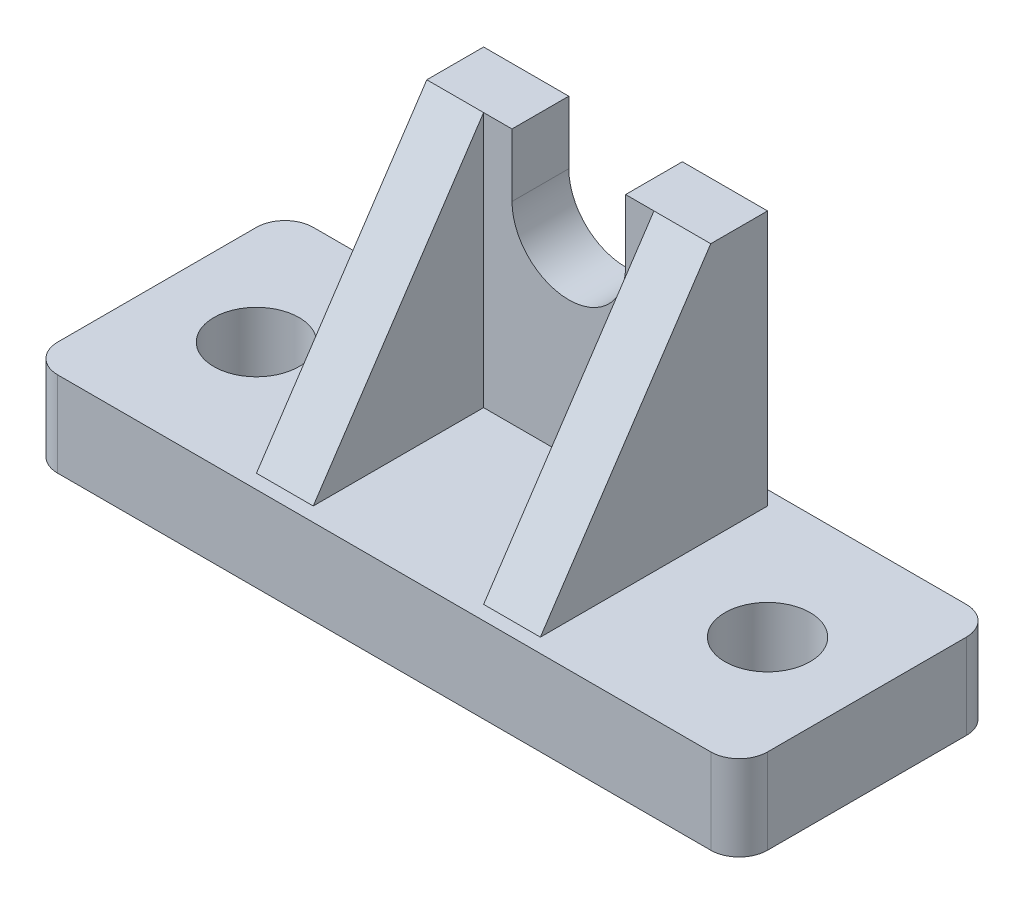
ISO-10303-21;
HEADER;
FILE_DESCRIPTION(('STEP AP214'),'2;1');
FILE_NAME('part.step','',(''),(''),'','','');
FILE_SCHEMA(('AUTOMOTIVE_DESIGN { 1 0 10303 214 1 1 1 1 }'));
ENDSEC;
DATA;
#1=APPLICATION_CONTEXT('core data for automotive mechanical design processes');
#2=APPLICATION_PROTOCOL_DEFINITION('international standard','automotive_design',2000,#1);
#3=PRODUCT_CONTEXT('',#1,'mechanical');
#4=PRODUCT('Part','Part','',(#3));
#5=PRODUCT_RELATED_PRODUCT_CATEGORY('part','',(#4));
#6=PRODUCT_DEFINITION_FORMATION('','',#4);
#7=PRODUCT_DEFINITION_CONTEXT('part definition',#1,'design');
#8=PRODUCT_DEFINITION('design','',#6,#7);
#9=PRODUCT_DEFINITION_SHAPE('','',#8);
#10=(LENGTH_UNIT() NAMED_UNIT(*) SI_UNIT(.MILLI.,.METRE.));
#11=(NAMED_UNIT(*) PLANE_ANGLE_UNIT() SI_UNIT($,.RADIAN.));
#12=(NAMED_UNIT(*) SI_UNIT($,.STERADIAN.) SOLID_ANGLE_UNIT());
#13=UNCERTAINTY_MEASURE_WITH_UNIT(LENGTH_MEASURE(1.E-05),#10,'distance_accuracy_value','');
#14=(GEOMETRIC_REPRESENTATION_CONTEXT(3) GLOBAL_UNCERTAINTY_ASSIGNED_CONTEXT((#13)) GLOBAL_UNIT_ASSIGNED_CONTEXT((#10,
#11,#12)) REPRESENTATION_CONTEXT('',''));
#15=CARTESIAN_POINT('',(0.,0.,0.));
#16=DIRECTION('',(0.,0.,1.));
#17=DIRECTION('',(1.,0.,0.));
#18=AXIS2_PLACEMENT_3D('',#15,#16,#17);
#19=CARTESIAN_POINT('',(50.,48.,-8.));
#20=DIRECTION('',(0.,-0.554700196225229,-0.832050294337844));
#21=DIRECTION('',(0.,0.832050294337844,-0.554700196225229));
#22=AXIS2_PLACEMENT_3D('',#19,#20,#21);
#23=PLANE('',#22);
#24=DIRECTION('',(0.,-0.832050294337844,0.554700196225229));
#25=VECTOR('',#24,1.);
#26=CARTESIAN_POINT('',(-12.,12.,16.));
#27=LINE('',#26,#25);
#28=CARTESIAN_POINT('',(-12.,48.,-8.));
#29=VERTEX_POINT('',#28);
#30=CARTESIAN_POINT('',(-12.,12.,16.));
#31=VERTEX_POINT('',#30);
#32=EDGE_CURVE('E181',#29,#31,#27,.T.);
#33=ORIENTED_EDGE('',*,*,#32,.F.);
#34=DIRECTION('',(-1.,0.,0.));
#35=VECTOR('',#34,1.);
#36=CARTESIAN_POINT('',(50.,48.,-8.));
#37=LINE('',#36,#35);
#38=CARTESIAN_POINT('',(-20.,48.,-8.));
#39=VERTEX_POINT('',#38);
#40=EDGE_CURVE('E197',#29,#39,#37,.T.);
#41=ORIENTED_EDGE('',*,*,#40,.T.);
#42=DIRECTION('',(0.,-0.832050294337844,0.554700196225229));
#43=VECTOR('',#42,1.);
#44=CARTESIAN_POINT('',(-20.,48.,-8.));
#45=LINE('',#44,#43);
#46=CARTESIAN_POINT('',(-20.,12.,16.));
#47=VERTEX_POINT('',#46);
#48=EDGE_CURVE('E194',#39,#47,#45,.T.);
#49=ORIENTED_EDGE('',*,*,#48,.T.);
#50=DIRECTION('',(-1.,0.,0.));
#51=VECTOR('',#50,1.);
#52=CARTESIAN_POINT('',(50.,12.,16.));
#53=LINE('',#52,#51);
#54=EDGE_CURVE('E178',#31,#47,#53,.T.);
#55=ORIENTED_EDGE('',*,*,#54,.F.);
#56=EDGE_LOOP('',(#33,#41,#49,#55));
#57=FACE_BOUND('',#56,.T.);
#58=ADVANCED_FACE('F39',(#57),#23,.F.);
#59=CARTESIAN_POINT('',(50.,12.,18.));
#60=DIRECTION('',(0.,-1.,0.));
#61=DIRECTION('',(1.,0.,0.));
#62=AXIS2_PLACEMENT_3D('',#59,#60,#61);
#63=PLANE('',#62);
#64=DIRECTION('',(-1.,0.,0.));
#65=VECTOR('',#64,1.);
#66=CARTESIAN_POINT('',(50.,12.,18.));
#67=LINE('',#66,#65);
#68=CARTESIAN_POINT('',(46.,12.,18.));
#69=VERTEX_POINT('',#68);
#70=CARTESIAN_POINT('',(-46.,12.,18.));
#71=VERTEX_POINT('',#70);
#72=EDGE_CURVE('E297',#69,#71,#67,.T.);
#73=ORIENTED_EDGE('',*,*,#72,.F.);
#74=CARTESIAN_POINT('',(46.,12.,14.));
#75=DIRECTION('',(0.,-1.,0.));
#76=DIRECTION('',(1.,0.,0.));
#77=AXIS2_PLACEMENT_3D('',#74,#75,#76);
#78=CIRCLE('',#77,4.);
#79=CARTESIAN_POINT('',(50.,12.,14.));
#80=VERTEX_POINT('',#79);
#81=EDGE_CURVE('E62',#80,#69,#78,.T.);
#82=ORIENTED_EDGE('',*,*,#81,.F.);
#83=DIRECTION('',(0.,0.,-1.));
#84=VECTOR('',#83,1.);
#85=CARTESIAN_POINT('',(50.,12.,18.));
#86=LINE('',#85,#84);
#87=CARTESIAN_POINT('',(50.,12.,-14.));
#88=VERTEX_POINT('',#87);
#89=EDGE_CURVE('E309',#80,#88,#86,.T.);
#90=ORIENTED_EDGE('',*,*,#89,.T.);
#91=CARTESIAN_POINT('',(46.,12.,-14.));
#92=DIRECTION('',(0.,-1.,0.));
#93=DIRECTION('',(-1.,0.,0.));
#94=AXIS2_PLACEMENT_3D('',#91,#92,#93);
#95=CIRCLE('',#94,4.);
#96=CARTESIAN_POINT('',(46.,12.,-18.));
#97=VERTEX_POINT('',#96);
#98=EDGE_CURVE('E268',#97,#88,#95,.T.);
#99=ORIENTED_EDGE('',*,*,#98,.F.);
#100=DIRECTION('',(-1.,0.,0.));
#101=VECTOR('',#100,1.);
#102=CARTESIAN_POINT('',(50.,12.,-18.));
#103=LINE('',#102,#101);
#104=CARTESIAN_POINT('',(-46.,12.,-18.));
#105=VERTEX_POINT('',#104);
#106=EDGE_CURVE('E299',#97,#105,#103,.T.);
#107=ORIENTED_EDGE('',*,*,#106,.T.);
#108=CARTESIAN_POINT('',(-46.,12.,-14.));
#109=DIRECTION('',(0.,-1.,0.));
#110=DIRECTION('',(1.,0.,0.));
#111=AXIS2_PLACEMENT_3D('',#108,#109,#110);
#112=CIRCLE('',#111,4.);
#113=CARTESIAN_POINT('',(-50.,12.,-14.));
#114=VERTEX_POINT('',#113);
#115=EDGE_CURVE('E262',#114,#105,#112,.T.);
#116=ORIENTED_EDGE('',*,*,#115,.F.);
#117=DIRECTION('',(0.,0.,-1.));
#118=VECTOR('',#117,1.);
#119=CARTESIAN_POINT('',(-50.,12.,18.));
#120=LINE('',#119,#118);
#121=CARTESIAN_POINT('',(-50.,12.,14.));
#122=VERTEX_POINT('',#121);
#123=EDGE_CURVE('E307',#122,#114,#120,.T.);
#124=ORIENTED_EDGE('',*,*,#123,.F.);
#125=CARTESIAN_POINT('',(-46.,12.,14.));
#126=DIRECTION('',(0.,-1.,0.));
#127=DIRECTION('',(-1.,0.,0.));
#128=AXIS2_PLACEMENT_3D('',#125,#126,#127);
#129=CIRCLE('',#128,4.);
#130=EDGE_CURVE('E267',#71,#122,#129,.T.);
#131=ORIENTED_EDGE('',*,*,#130,.F.);
#132=EDGE_LOOP('',(#73,#82,#90,#99,#107,#116,#124,#131));
#133=FACE_BOUND('',#132,.T.);
#134=CARTESIAN_POINT('',(36.,12.,0.));
#135=DIRECTION('',(0.,1.,0.));
#136=DIRECTION('',(1.,0.,0.));
#137=AXIS2_PLACEMENT_3D('',#134,#135,#136);
#138=CIRCLE('',#137,6.);
#139=CARTESIAN_POINT('',(42.,12.,0.));
#140=VERTEX_POINT('',#139);
#141=EDGE_CURVE('E235',#140,#140,#138,.T.);
#142=ORIENTED_EDGE('',*,*,#141,.F.);
#143=EDGE_LOOP('',(#142));
#144=FACE_BOUND('',#143,.T.);
#145=CARTESIAN_POINT('',(-36.,12.,0.));
#146=DIRECTION('',(0.,1.,0.));
#147=DIRECTION('',(-1.,0.,0.));
#148=AXIS2_PLACEMENT_3D('',#145,#146,#147);
#149=CIRCLE('',#148,6.);
#150=CARTESIAN_POINT('',(-42.,12.,0.));
#151=VERTEX_POINT('',#150);
#152=EDGE_CURVE('E251',#151,#151,#149,.T.);
#153=ORIENTED_EDGE('',*,*,#152,.F.);
#154=EDGE_LOOP('',(#153));
#155=FACE_BOUND('',#154,.T.);
#156=DIRECTION('',(0.,0.,1.));
#157=VECTOR('',#156,1.);
#158=CARTESIAN_POINT('',(20.,12.,-16.));
#159=LINE('',#158,#157);
#160=CARTESIAN_POINT('',(20.,12.,-16.));
#161=VERTEX_POINT('',#160);
#162=CARTESIAN_POINT('',(20.,12.,16.));
#163=VERTEX_POINT('',#162);
#164=EDGE_CURVE('E241',#161,#163,#159,.T.);
#165=ORIENTED_EDGE('',*,*,#164,.T.);
#166=CARTESIAN_POINT('',(12.,12.,16.));
#167=VERTEX_POINT('',#166);
#168=EDGE_CURVE('E195',#163,#167,#53,.T.);
#169=ORIENTED_EDGE('',*,*,#168,.T.);
#170=DIRECTION('',(0.,0.,-1.));
#171=VECTOR('',#170,1.);
#172=CARTESIAN_POINT('',(12.,12.,-8.));
#173=LINE('',#172,#171);
#174=CARTESIAN_POINT('',(12.,12.,-8.));
#175=VERTEX_POINT('',#174);
#176=EDGE_CURVE('E53',#167,#175,#173,.T.);
#177=ORIENTED_EDGE('',*,*,#176,.T.);
#178=DIRECTION('',(1.,0.,0.));
#179=VECTOR('',#178,1.);
#180=CARTESIAN_POINT('',(-12.,12.,-8.));
#181=LINE('',#180,#179);
#182=CARTESIAN_POINT('',(-12.,12.,-8.));
#183=VERTEX_POINT('',#182);
#184=EDGE_CURVE('E177',#183,#175,#181,.T.);
#185=ORIENTED_EDGE('',*,*,#184,.F.);
#186=DIRECTION('',(0.,0.,-1.));
#187=VECTOR('',#186,1.);
#188=CARTESIAN_POINT('',(-12.,12.,-8.));
#189=LINE('',#188,#187);
#190=EDGE_CURVE('E168',#31,#183,#189,.T.);
#191=ORIENTED_EDGE('',*,*,#190,.F.);
#192=ORIENTED_EDGE('',*,*,#54,.T.);
#193=DIRECTION('',(0.,0.,1.));
#194=VECTOR('',#193,1.);
#195=CARTESIAN_POINT('',(-20.,12.,-16.));
#196=LINE('',#195,#194);
#197=CARTESIAN_POINT('',(-20.,12.,-16.));
#198=VERTEX_POINT('',#197);
#199=EDGE_CURVE('E244',#198,#47,#196,.T.);
#200=ORIENTED_EDGE('',*,*,#199,.F.);
#201=DIRECTION('',(1.,0.,0.));
#202=VECTOR('',#201,1.);
#203=CARTESIAN_POINT('',(-20.,12.,-16.));
#204=LINE('',#203,#202);
#205=EDGE_CURVE('E217',#198,#161,#204,.T.);
#206=ORIENTED_EDGE('',*,*,#205,.T.);
#207=EDGE_LOOP('',(#165,#169,#177,#185,#191,#192,#200,#206));
#208=FACE_BOUND('',#207,.T.);
#209=ADVANCED_FACE('F174',(#133,#144,#155,#208),#63,.F.);
#210=CARTESIAN_POINT('',(50.,0.,18.));
#211=DIRECTION('',(-1.,0.,0.));
#212=DIRECTION('',(0.,0.,1.));
#213=AXIS2_PLACEMENT_3D('',#210,#211,#212);
#214=PLANE('',#213);
#215=DIRECTION('',(0.,1.,0.));
#216=VECTOR('',#215,1.);
#217=CARTESIAN_POINT('',(50.,-24.,-14.));
#218=LINE('',#217,#216);
#219=CARTESIAN_POINT('',(50.,0.,-14.));
#220=VERTEX_POINT('',#219);
#221=EDGE_CURVE('E275',#220,#88,#218,.T.);
#222=ORIENTED_EDGE('',*,*,#221,.T.);
#223=ORIENTED_EDGE('',*,*,#89,.F.);
#224=DIRECTION('',(0.,1.,0.));
#225=VECTOR('',#224,1.);
#226=CARTESIAN_POINT('',(50.,-24.,14.));
#227=LINE('',#226,#225);
#228=CARTESIAN_POINT('',(50.,0.,14.));
#229=VERTEX_POINT('',#228);
#230=EDGE_CURVE('E276',#229,#80,#227,.T.);
#231=ORIENTED_EDGE('',*,*,#230,.F.);
#232=DIRECTION('',(0.,0.,-1.));
#233=VECTOR('',#232,1.);
#234=CARTESIAN_POINT('',(50.,0.,18.));
#235=LINE('',#234,#233);
#236=EDGE_CURVE('E311',#229,#220,#235,.T.);
#237=ORIENTED_EDGE('',*,*,#236,.T.);
#238=EDGE_LOOP('',(#222,#223,#231,#237));
#239=FACE_BOUND('',#238,.T.);
#240=ADVANCED_FACE('F351',(#239),#214,.F.);
#241=CARTESIAN_POINT('',(-50.,12.,18.));
#242=DIRECTION('',(1.,0.,0.));
#243=DIRECTION('',(0.,0.,-1.));
#244=AXIS2_PLACEMENT_3D('',#241,#242,#243);
#245=PLANE('',#244);
#246=DIRECTION('',(0.,1.,0.));
#247=VECTOR('',#246,1.);
#248=CARTESIAN_POINT('',(-50.,-24.,14.));
#249=LINE('',#248,#247);
#250=CARTESIAN_POINT('',(-50.,0.,14.));
#251=VERTEX_POINT('',#250);
#252=EDGE_CURVE('E271',#251,#122,#249,.T.);
#253=ORIENTED_EDGE('',*,*,#252,.T.);
#254=ORIENTED_EDGE('',*,*,#123,.T.);
#255=DIRECTION('',(0.,1.,0.));
#256=VECTOR('',#255,1.);
#257=CARTESIAN_POINT('',(-50.,-24.,-14.));
#258=LINE('',#257,#256);
#259=CARTESIAN_POINT('',(-50.,0.,-14.));
#260=VERTEX_POINT('',#259);
#261=EDGE_CURVE('E266',#260,#114,#258,.T.);
#262=ORIENTED_EDGE('',*,*,#261,.F.);
#263=DIRECTION('',(0.,0.,-1.));
#264=VECTOR('',#263,1.);
#265=CARTESIAN_POINT('',(-50.,0.,18.));
#266=LINE('',#265,#264);
#267=EDGE_CURVE('E300',#251,#260,#266,.T.);
#268=ORIENTED_EDGE('',*,*,#267,.F.);
#269=EDGE_LOOP('',(#253,#254,#262,#268));
#270=FACE_BOUND('',#269,.T.);
#271=ADVANCED_FACE('F339',(#270),#245,.F.);
#272=CARTESIAN_POINT('',(0.,0.,18.));
#273=DIRECTION('',(0.,0.,1.));
#274=DIRECTION('',(1.,0.,0.));
#275=AXIS2_PLACEMENT_3D('',#272,#273,#274);
#276=PLANE('',#275);
#277=ORIENTED_EDGE('',*,*,#72,.T.);
#278=DIRECTION('',(0.,1.,0.));
#279=VECTOR('',#278,1.);
#280=CARTESIAN_POINT('',(-46.,-24.,18.));
#281=LINE('',#280,#279);
#282=CARTESIAN_POINT('',(-46.,0.,18.));
#283=VERTEX_POINT('',#282);
#284=EDGE_CURVE('E11',#71,#283,#281,.F.);
#285=ORIENTED_EDGE('',*,*,#284,.T.);
#286=DIRECTION('',(1.,0.,0.));
#287=VECTOR('',#286,1.);
#288=CARTESIAN_POINT('',(-50.,0.,18.));
#289=LINE('',#288,#287);
#290=CARTESIAN_POINT('',(46.,0.,18.));
#291=VERTEX_POINT('',#290);
#292=EDGE_CURVE('E294',#283,#291,#289,.T.);
#293=ORIENTED_EDGE('',*,*,#292,.T.);
#294=DIRECTION('',(0.,1.,0.));
#295=VECTOR('',#294,1.);
#296=CARTESIAN_POINT('',(46.,-24.,18.));
#297=LINE('',#296,#295);
#298=EDGE_CURVE('E50',#69,#291,#297,.F.);
#299=ORIENTED_EDGE('',*,*,#298,.F.);
#300=EDGE_LOOP('',(#277,#285,#293,#299));
#301=FACE_BOUND('',#300,.T.);
#302=ADVANCED_FACE('F330',(#301),#276,.T.);
#303=CARTESIAN_POINT('',(0.,0.,-18.));
#304=DIRECTION('',(0.,0.,1.));
#305=DIRECTION('',(1.,0.,0.));
#306=AXIS2_PLACEMENT_3D('',#303,#304,#305);
#307=PLANE('',#306);
#308=ORIENTED_EDGE('',*,*,#106,.F.);
#309=DIRECTION('',(0.,1.,0.));
#310=VECTOR('',#309,1.);
#311=CARTESIAN_POINT('',(46.,-24.,-18.));
#312=LINE('',#311,#310);
#313=CARTESIAN_POINT('',(46.,0.,-18.));
#314=VERTEX_POINT('',#313);
#315=EDGE_CURVE('E318',#97,#314,#312,.F.);
#316=ORIENTED_EDGE('',*,*,#315,.T.);
#317=DIRECTION('',(1.,0.,0.));
#318=VECTOR('',#317,1.);
#319=CARTESIAN_POINT('',(0.,0.,-18.));
#320=LINE('',#319,#318);
#321=CARTESIAN_POINT('',(-46.,0.,-18.));
#322=VERTEX_POINT('',#321);
#323=EDGE_CURVE('E291',#322,#314,#320,.T.);
#324=ORIENTED_EDGE('',*,*,#323,.F.);
#325=DIRECTION('',(0.,1.,0.));
#326=VECTOR('',#325,1.);
#327=CARTESIAN_POINT('',(-46.,-24.,-18.));
#328=LINE('',#327,#326);
#329=EDGE_CURVE('E316',#105,#322,#328,.F.);
#330=ORIENTED_EDGE('',*,*,#329,.F.);
#331=EDGE_LOOP('',(#308,#316,#324,#330));
#332=FACE_BOUND('',#331,.T.);
#333=ADVANCED_FACE('F341',(#332),#307,.F.);
#334=CARTESIAN_POINT('',(0.,0.,18.));
#335=DIRECTION('',(0.,1.,0.));
#336=DIRECTION('',(0.,0.,1.));
#337=AXIS2_PLACEMENT_3D('',#334,#335,#336);
#338=PLANE('',#337);
#339=CARTESIAN_POINT('',(-36.,0.,0.));
#340=DIRECTION('',(0.,1.,0.));
#341=DIRECTION('',(0.,0.,1.));
#342=AXIS2_PLACEMENT_3D('',#339,#340,#341);
#343=CIRCLE('',#342,6.);
#344=CARTESIAN_POINT('',(-36.,0.,6.));
#345=VERTEX_POINT('',#344);
#346=EDGE_CURVE('E261',#345,#345,#343,.T.);
#347=ORIENTED_EDGE('',*,*,#346,.T.);
#348=EDGE_LOOP('',(#347));
#349=FACE_BOUND('',#348,.T.);
#350=CARTESIAN_POINT('',(36.,0.,0.));
#351=DIRECTION('',(0.,1.,0.));
#352=DIRECTION('',(0.,0.,1.));
#353=AXIS2_PLACEMENT_3D('',#350,#351,#352);
#354=CIRCLE('',#353,6.);
#355=CARTESIAN_POINT('',(36.,0.,6.));
#356=VERTEX_POINT('',#355);
#357=EDGE_CURVE('E258',#356,#356,#354,.T.);
#358=ORIENTED_EDGE('',*,*,#357,.T.);
#359=EDGE_LOOP('',(#358));
#360=FACE_BOUND('',#359,.T.);
#361=ORIENTED_EDGE('',*,*,#292,.F.);
#362=CARTESIAN_POINT('',(-46.,0.,14.));
#363=DIRECTION('',(0.,1.,0.));
#364=DIRECTION('',(0.,0.,1.));
#365=AXIS2_PLACEMENT_3D('',#362,#363,#364);
#366=CIRCLE('',#365,4.);
#367=EDGE_CURVE('E286',#283,#251,#366,.F.);
#368=ORIENTED_EDGE('',*,*,#367,.T.);
#369=ORIENTED_EDGE('',*,*,#267,.T.);
#370=CARTESIAN_POINT('',(-46.,0.,-14.));
#371=DIRECTION('',(0.,1.,0.));
#372=DIRECTION('',(0.,0.,1.));
#373=AXIS2_PLACEMENT_3D('',#370,#371,#372);
#374=CIRCLE('',#373,4.);
#375=EDGE_CURVE('E281',#260,#322,#374,.F.);
#376=ORIENTED_EDGE('',*,*,#375,.T.);
#377=ORIENTED_EDGE('',*,*,#323,.T.);
#378=CARTESIAN_POINT('',(46.,0.,-14.));
#379=DIRECTION('',(0.,1.,0.));
#380=DIRECTION('',(0.,0.,1.));
#381=AXIS2_PLACEMENT_3D('',#378,#379,#380);
#382=CIRCLE('',#381,4.);
#383=EDGE_CURVE('E283',#314,#220,#382,.F.);
#384=ORIENTED_EDGE('',*,*,#383,.T.);
#385=ORIENTED_EDGE('',*,*,#236,.F.);
#386=CARTESIAN_POINT('',(46.,0.,14.));
#387=DIRECTION('',(0.,1.,0.));
#388=DIRECTION('',(0.,0.,1.));
#389=AXIS2_PLACEMENT_3D('',#386,#387,#388);
#390=CIRCLE('',#389,4.);
#391=EDGE_CURVE('E289',#229,#291,#390,.F.);
#392=ORIENTED_EDGE('',*,*,#391,.T.);
#393=EDGE_LOOP('',(#361,#368,#369,#376,#377,#384,#385,#392));
#394=FACE_BOUND('',#393,.T.);
#395=ADVANCED_FACE('F41',(#349,#360,#394),#338,.F.);
#396=CARTESIAN_POINT('',(-46.,-24.,-14.));
#397=DIRECTION('',(0.,1.,0.));
#398=DIRECTION('',(-1.,0.,0.));
#399=AXIS2_PLACEMENT_3D('',#396,#397,#398);
#400=CYLINDRICAL_SURFACE('',#399,4.);
#401=ORIENTED_EDGE('',*,*,#261,.T.);
#402=ORIENTED_EDGE('',*,*,#115,.T.);
#403=ORIENTED_EDGE('',*,*,#329,.T.);
#404=ORIENTED_EDGE('',*,*,#375,.F.);
#405=EDGE_LOOP('',(#401,#402,#403,#404));
#406=FACE_BOUND('',#405,.T.);
#407=ADVANCED_FACE('F547',(#406),#400,.T.);
#408=CARTESIAN_POINT('',(46.,-24.,-14.));
#409=DIRECTION('',(0.,1.,0.));
#410=DIRECTION('',(-1.,0.,0.));
#411=AXIS2_PLACEMENT_3D('',#408,#409,#410);
#412=CYLINDRICAL_SURFACE('',#411,4.);
#413=ORIENTED_EDGE('',*,*,#315,.F.);
#414=ORIENTED_EDGE('',*,*,#98,.T.);
#415=ORIENTED_EDGE('',*,*,#221,.F.);
#416=ORIENTED_EDGE('',*,*,#383,.F.);
#417=EDGE_LOOP('',(#413,#414,#415,#416));
#418=FACE_BOUND('',#417,.T.);
#419=ADVANCED_FACE('F346',(#418),#412,.T.);
#420=CARTESIAN_POINT('',(46.,-24.,14.));
#421=DIRECTION('',(0.,1.,0.));
#422=DIRECTION('',(-1.,0.,0.));
#423=AXIS2_PLACEMENT_3D('',#420,#421,#422);
#424=CYLINDRICAL_SURFACE('',#423,4.);
#425=ORIENTED_EDGE('',*,*,#230,.T.);
#426=ORIENTED_EDGE('',*,*,#81,.T.);
#427=ORIENTED_EDGE('',*,*,#298,.T.);
#428=ORIENTED_EDGE('',*,*,#391,.F.);
#429=EDGE_LOOP('',(#425,#426,#427,#428));
#430=FACE_BOUND('',#429,.T.);
#431=ADVANCED_FACE('F319',(#430),#424,.T.);
#432=CARTESIAN_POINT('',(-46.,-24.,14.));
#433=DIRECTION('',(0.,1.,0.));
#434=DIRECTION('',(-1.,0.,0.));
#435=AXIS2_PLACEMENT_3D('',#432,#433,#434);
#436=CYLINDRICAL_SURFACE('',#435,4.);
#437=ORIENTED_EDGE('',*,*,#284,.F.);
#438=ORIENTED_EDGE('',*,*,#130,.T.);
#439=ORIENTED_EDGE('',*,*,#252,.F.);
#440=ORIENTED_EDGE('',*,*,#367,.F.);
#441=EDGE_LOOP('',(#437,#438,#439,#440));
#442=FACE_BOUND('',#441,.T.);
#443=ADVANCED_FACE('F332',(#442),#436,.T.);
#444=CARTESIAN_POINT('',(36.,-24.,0.));
#445=DIRECTION('',(0.,1.,0.));
#446=DIRECTION('',(-1.,0.,0.));
#447=AXIS2_PLACEMENT_3D('',#444,#445,#446);
#448=CYLINDRICAL_SURFACE('',#447,6.);
#449=ORIENTED_EDGE('',*,*,#141,.T.);
#450=EDGE_LOOP('',(#449));
#451=FACE_BOUND('',#450,.T.);
#452=ORIENTED_EDGE('',*,*,#357,.F.);
#453=EDGE_LOOP('',(#452));
#454=FACE_BOUND('',#453,.T.);
#455=ADVANCED_FACE('F517',(#451,#454),#448,.F.);
#456=CARTESIAN_POINT('',(-36.,-24.,0.));
#457=DIRECTION('',(0.,1.,0.));
#458=DIRECTION('',(-1.,0.,0.));
#459=AXIS2_PLACEMENT_3D('',#456,#457,#458);
#460=CYLINDRICAL_SURFACE('',#459,6.);
#461=ORIENTED_EDGE('',*,*,#152,.T.);
#462=EDGE_LOOP('',(#461));
#463=FACE_BOUND('',#462,.T.);
#464=ORIENTED_EDGE('',*,*,#346,.F.);
#465=EDGE_LOOP('',(#464));
#466=FACE_BOUND('',#465,.T.);
#467=ADVANCED_FACE('F504',(#463,#466),#460,.F.);
#468=CARTESIAN_POINT('',(0.,39.1509513170679,-16.));
#469=DIRECTION('',(0.,0.,1.));
#470=DIRECTION('',(1.,0.,0.));
#471=AXIS2_PLACEMENT_3D('',#468,#469,#470);
#472=CYLINDRICAL_SURFACE('',#471,7.99999999999999);
#473=CARTESIAN_POINT('',(0.,39.1509513170679,-8.));
#474=DIRECTION('',(0.,0.,-1.));
#475=DIRECTION('',(-1.,0.,0.));
#476=AXIS2_PLACEMENT_3D('',#473,#474,#475);
#477=CIRCLE('',#476,7.99999999999999);
#478=CARTESIAN_POINT('',(7.99999999999999,39.1509513170679,-8.));
#479=VERTEX_POINT('',#478);
#480=CARTESIAN_POINT('',(-8.,39.1509513170679,-8.));
#481=VERTEX_POINT('',#480);
#482=EDGE_CURVE('E402',#479,#481,#477,.T.);
#483=ORIENTED_EDGE('',*,*,#482,.F.);
#484=DIRECTION('',(0.,0.,1.));
#485=VECTOR('',#484,1.);
#486=CARTESIAN_POINT('',(7.99999999999999,39.1509513170679,-16.));
#487=LINE('',#486,#485);
#488=CARTESIAN_POINT('',(7.99999999999999,39.1509513170679,-16.));
#489=VERTEX_POINT('',#488);
#490=EDGE_CURVE('E233',#489,#479,#487,.T.);
#491=ORIENTED_EDGE('',*,*,#490,.F.);
#492=CARTESIAN_POINT('',(0.,39.1509513170679,-16.));
#493=DIRECTION('',(0.,0.,-1.));
#494=DIRECTION('',(-1.,0.,0.));
#495=AXIS2_PLACEMENT_3D('',#492,#493,#494);
#496=CIRCLE('',#495,7.99999999999999);
#497=CARTESIAN_POINT('',(-8.,39.1509513170679,-16.));
#498=VERTEX_POINT('',#497);
#499=EDGE_CURVE('E202',#489,#498,#496,.T.);
#500=ORIENTED_EDGE('',*,*,#499,.T.);
#501=DIRECTION('',(0.,0.,1.));
#502=VECTOR('',#501,1.);
#503=CARTESIAN_POINT('',(-8.,39.1509513170679,-16.));
#504=LINE('',#503,#502);
#505=EDGE_CURVE('E230',#498,#481,#504,.T.);
#506=ORIENTED_EDGE('',*,*,#505,.T.);
#507=EDGE_LOOP('',(#483,#491,#500,#506));
#508=FACE_BOUND('',#507,.T.);
#509=ADVANCED_FACE('F396',(#508),#472,.F.);
#510=CARTESIAN_POINT('',(7.99999999999999,39.1509513170679,-16.));
#511=DIRECTION('',(-1.,0.,0.));
#512=DIRECTION('',(0.,-1.,0.));
#513=AXIS2_PLACEMENT_3D('',#510,#511,#512);
#514=PLANE('',#513);
#515=DIRECTION('',(0.,-1.,0.));
#516=VECTOR('',#515,1.);
#517=CARTESIAN_POINT('',(7.99999999999999,39.1509513170679,-8.));
#518=LINE('',#517,#516);
#519=CARTESIAN_POINT('',(7.99999999999999,48.,-8.));
#520=VERTEX_POINT('',#519);
#521=EDGE_CURVE('E196',#520,#479,#518,.T.);
#522=ORIENTED_EDGE('',*,*,#521,.F.);
#523=DIRECTION('',(0.,0.,1.));
#524=VECTOR('',#523,1.);
#525=CARTESIAN_POINT('',(7.99999999999999,48.,-16.));
#526=LINE('',#525,#524);
#527=CARTESIAN_POINT('',(7.99999999999999,48.,-16.));
#528=VERTEX_POINT('',#527);
#529=EDGE_CURVE('E231',#528,#520,#526,.T.);
#530=ORIENTED_EDGE('',*,*,#529,.F.);
#531=DIRECTION('',(0.,-1.,0.));
#532=VECTOR('',#531,1.);
#533=CARTESIAN_POINT('',(7.99999999999999,39.1509513170679,-16.));
#534=LINE('',#533,#532);
#535=EDGE_CURVE('E227',#528,#489,#534,.T.);
#536=ORIENTED_EDGE('',*,*,#535,.T.);
#537=ORIENTED_EDGE('',*,*,#490,.T.);
#538=EDGE_LOOP('',(#522,#530,#536,#537));
#539=FACE_BOUND('',#538,.T.);
#540=ADVANCED_FACE('F406',(#539),#514,.T.);
#541=CARTESIAN_POINT('',(7.99999999999999,48.,-16.));
#542=DIRECTION('',(0.,1.,0.));
#543=DIRECTION('',(-1.,0.,0.));
#544=AXIS2_PLACEMENT_3D('',#541,#542,#543);
#545=PLANE('',#544);
#546=CARTESIAN_POINT('',(20.,48.,-8.));
#547=VERTEX_POINT('',#546);
#548=CARTESIAN_POINT('',(12.,48.,-8.));
#549=VERTEX_POINT('',#548);
#550=EDGE_CURVE('E206',#547,#549,#37,.T.);
#551=ORIENTED_EDGE('',*,*,#550,.F.);
#552=DIRECTION('',(0.,0.,1.));
#553=VECTOR('',#552,1.);
#554=CARTESIAN_POINT('',(20.,48.,-16.));
#555=LINE('',#554,#553);
#556=CARTESIAN_POINT('',(20.,48.,-16.));
#557=VERTEX_POINT('',#556);
#558=EDGE_CURVE('E236',#557,#547,#555,.T.);
#559=ORIENTED_EDGE('',*,*,#558,.F.);
#560=DIRECTION('',(-1.,0.,0.));
#561=VECTOR('',#560,1.);
#562=CARTESIAN_POINT('',(7.99999999999999,48.,-16.));
#563=LINE('',#562,#561);
#564=EDGE_CURVE('E221',#557,#528,#563,.T.);
#565=ORIENTED_EDGE('',*,*,#564,.T.);
#566=ORIENTED_EDGE('',*,*,#529,.T.);
#567=EDGE_CURVE('E384',#549,#520,#37,.T.);
#568=ORIENTED_EDGE('',*,*,#567,.F.);
#569=EDGE_LOOP('',(#551,#559,#565,#566,#568));
#570=FACE_BOUND('',#569,.T.);
#571=ADVANCED_FACE('F407',(#570),#545,.T.);
#572=CARTESIAN_POINT('',(20.,48.,-16.));
#573=DIRECTION('',(1.,0.,0.));
#574=DIRECTION('',(0.,1.,0.));
#575=AXIS2_PLACEMENT_3D('',#572,#573,#574);
#576=PLANE('',#575);
#577=DIRECTION('',(0.,0.832050294337844,-0.554700196225229));
#578=VECTOR('',#577,1.);
#579=CARTESIAN_POINT('',(20.,51.6923076923077,-10.4615384615385));
#580=LINE('',#579,#578);
#581=EDGE_CURVE('E201',#163,#547,#580,.T.);
#582=ORIENTED_EDGE('',*,*,#581,.F.);
#583=ORIENTED_EDGE('',*,*,#164,.F.);
#584=DIRECTION('',(0.,1.,0.));
#585=VECTOR('',#584,1.);
#586=CARTESIAN_POINT('',(20.,48.,-16.));
#587=LINE('',#586,#585);
#588=EDGE_CURVE('E222',#161,#557,#587,.T.);
#589=ORIENTED_EDGE('',*,*,#588,.T.);
#590=ORIENTED_EDGE('',*,*,#558,.T.);
#591=EDGE_LOOP('',(#582,#583,#589,#590));
#592=FACE_BOUND('',#591,.T.);
#593=ADVANCED_FACE('F410',(#592),#576,.T.);
#594=CARTESIAN_POINT('',(-20.,48.,-16.));
#595=DIRECTION('',(-1.,0.,0.));
#596=DIRECTION('',(0.,-1.,0.));
#597=AXIS2_PLACEMENT_3D('',#594,#595,#596);
#598=PLANE('',#597);
#599=ORIENTED_EDGE('',*,*,#48,.F.);
#600=DIRECTION('',(0.,0.,1.));
#601=VECTOR('',#600,1.);
#602=CARTESIAN_POINT('',(-20.,48.,-16.));
#603=LINE('',#602,#601);
#604=CARTESIAN_POINT('',(-20.,48.,-16.));
#605=VERTEX_POINT('',#604);
#606=EDGE_CURVE('E245',#605,#39,#603,.T.);
#607=ORIENTED_EDGE('',*,*,#606,.F.);
#608=DIRECTION('',(0.,-1.,0.));
#609=VECTOR('',#608,1.);
#610=CARTESIAN_POINT('',(-20.,48.,-16.));
#611=LINE('',#610,#609);
#612=EDGE_CURVE('E214',#605,#198,#611,.T.);
#613=ORIENTED_EDGE('',*,*,#612,.T.);
#614=ORIENTED_EDGE('',*,*,#199,.T.);
#615=EDGE_LOOP('',(#599,#607,#613,#614));
#616=FACE_BOUND('',#615,.T.);
#617=ADVANCED_FACE('F386',(#616),#598,.T.);
#618=CARTESIAN_POINT('',(-8.,48.,-16.));
#619=DIRECTION('',(0.,1.,0.));
#620=DIRECTION('',(-1.,0.,0.));
#621=AXIS2_PLACEMENT_3D('',#618,#619,#620);
#622=PLANE('',#621);
#623=CARTESIAN_POINT('',(-8.,48.,-8.));
#624=VERTEX_POINT('',#623);
#625=EDGE_CURVE('E205',#624,#29,#37,.T.);
#626=ORIENTED_EDGE('',*,*,#625,.F.);
#627=DIRECTION('',(0.,0.,1.));
#628=VECTOR('',#627,1.);
#629=CARTESIAN_POINT('',(-8.,48.,-16.));
#630=LINE('',#629,#628);
#631=CARTESIAN_POINT('',(-8.,48.,-16.));
#632=VERTEX_POINT('',#631);
#633=EDGE_CURVE('E247',#632,#624,#630,.T.);
#634=ORIENTED_EDGE('',*,*,#633,.F.);
#635=DIRECTION('',(-1.,0.,0.));
#636=VECTOR('',#635,1.);
#637=CARTESIAN_POINT('',(-8.,48.,-16.));
#638=LINE('',#637,#636);
#639=EDGE_CURVE('E215',#632,#605,#638,.T.);
#640=ORIENTED_EDGE('',*,*,#639,.T.);
#641=ORIENTED_EDGE('',*,*,#606,.T.);
#642=ORIENTED_EDGE('',*,*,#40,.F.);
#643=EDGE_LOOP('',(#626,#634,#640,#641,#642));
#644=FACE_BOUND('',#643,.T.);
#645=ADVANCED_FACE('F391',(#644),#622,.T.);
#646=CARTESIAN_POINT('',(-8.,39.1509513170679,-16.));
#647=DIRECTION('',(1.,0.,0.));
#648=DIRECTION('',(0.,1.,0.));
#649=AXIS2_PLACEMENT_3D('',#646,#647,#648);
#650=PLANE('',#649);
#651=DIRECTION('',(0.,1.,0.));
#652=VECTOR('',#651,1.);
#653=CARTESIAN_POINT('',(-8.,39.1509513170679,-8.));
#654=LINE('',#653,#652);
#655=EDGE_CURVE('E399',#481,#624,#654,.T.);
#656=ORIENTED_EDGE('',*,*,#655,.F.);
#657=ORIENTED_EDGE('',*,*,#505,.F.);
#658=DIRECTION('',(0.,1.,0.));
#659=VECTOR('',#658,1.);
#660=CARTESIAN_POINT('',(-8.,39.1509513170679,-16.));
#661=LINE('',#660,#659);
#662=EDGE_CURVE('E207',#498,#632,#661,.T.);
#663=ORIENTED_EDGE('',*,*,#662,.T.);
#664=ORIENTED_EDGE('',*,*,#633,.T.);
#665=EDGE_LOOP('',(#656,#657,#663,#664));
#666=FACE_BOUND('',#665,.T.);
#667=ADVANCED_FACE('F380',(#666),#650,.T.);
#668=CARTESIAN_POINT('',(0.,39.1509513170679,-16.));
#669=DIRECTION('',(0.,0.,-1.));
#670=DIRECTION('',(-1.,0.,0.));
#671=AXIS2_PLACEMENT_3D('',#668,#669,#670);
#672=PLANE('',#671);
#673=ORIENTED_EDGE('',*,*,#499,.F.);
#674=ORIENTED_EDGE('',*,*,#535,.F.);
#675=ORIENTED_EDGE('',*,*,#564,.F.);
#676=ORIENTED_EDGE('',*,*,#588,.F.);
#677=ORIENTED_EDGE('',*,*,#205,.F.);
#678=ORIENTED_EDGE('',*,*,#612,.F.);
#679=ORIENTED_EDGE('',*,*,#639,.F.);
#680=ORIENTED_EDGE('',*,*,#662,.F.);
#681=EDGE_LOOP('',(#673,#674,#675,#676,#677,#678,#679,#680));
#682=FACE_BOUND('',#681,.T.);
#683=ADVANCED_FACE('F369',(#682),#672,.T.);
#684=ORIENTED_EDGE('',*,*,#550,.T.);
#685=DIRECTION('',(0.,-0.832050294337844,0.554700196225229));
#686=VECTOR('',#685,1.);
#687=CARTESIAN_POINT('',(12.,12.,16.));
#688=LINE('',#687,#686);
#689=EDGE_CURVE('E381',#549,#167,#688,.T.);
#690=ORIENTED_EDGE('',*,*,#689,.T.);
#691=ORIENTED_EDGE('',*,*,#168,.F.);
#692=ORIENTED_EDGE('',*,*,#581,.T.);
#693=EDGE_LOOP('',(#684,#690,#691,#692));
#694=FACE_BOUND('',#693,.T.);
#695=ADVANCED_FACE('F363',(#694),#23,.F.);
#696=CARTESIAN_POINT('',(-12.,48.,-8.));
#697=DIRECTION('',(0.,0.,-1.));
#698=DIRECTION('',(-1.,0.,0.));
#699=AXIS2_PLACEMENT_3D('',#696,#697,#698);
#700=PLANE('',#699);
#701=ORIENTED_EDGE('',*,*,#521,.T.);
#702=ORIENTED_EDGE('',*,*,#482,.T.);
#703=ORIENTED_EDGE('',*,*,#655,.T.);
#704=ORIENTED_EDGE('',*,*,#625,.T.);
#705=DIRECTION('',(0.,1.,0.));
#706=VECTOR('',#705,1.);
#707=CARTESIAN_POINT('',(-12.,48.,-8.));
#708=LINE('',#707,#706);
#709=EDGE_CURVE('E185',#183,#29,#708,.T.);
#710=ORIENTED_EDGE('',*,*,#709,.F.);
#711=ORIENTED_EDGE('',*,*,#184,.T.);
#712=DIRECTION('',(0.,1.,0.));
#713=VECTOR('',#712,1.);
#714=CARTESIAN_POINT('',(12.,48.,-8.));
#715=LINE('',#714,#713);
#716=EDGE_CURVE('E188',#175,#549,#715,.T.);
#717=ORIENTED_EDGE('',*,*,#716,.T.);
#718=ORIENTED_EDGE('',*,*,#567,.T.);
#719=EDGE_LOOP('',(#701,#702,#703,#704,#710,#711,#717,#718));
#720=FACE_BOUND('',#719,.T.);
#721=ADVANCED_FACE('F366',(#720),#700,.F.);
#722=CARTESIAN_POINT('',(-12.,0.,0.));
#723=DIRECTION('',(1.,0.,0.));
#724=DIRECTION('',(0.,0.,-1.));
#725=AXIS2_PLACEMENT_3D('',#722,#723,#724);
#726=PLANE('',#725);
#727=ORIENTED_EDGE('',*,*,#32,.T.);
#728=ORIENTED_EDGE('',*,*,#190,.T.);
#729=ORIENTED_EDGE('',*,*,#709,.T.);
#730=EDGE_LOOP('',(#727,#728,#729));
#731=FACE_BOUND('',#730,.T.);
#732=ADVANCED_FACE('F186',(#731),#726,.T.);
#733=CARTESIAN_POINT('',(12.,0.,0.));
#734=DIRECTION('',(1.,0.,0.));
#735=DIRECTION('',(0.,0.,-1.));
#736=AXIS2_PLACEMENT_3D('',#733,#734,#735);
#737=PLANE('',#736);
#738=ORIENTED_EDGE('',*,*,#689,.F.);
#739=ORIENTED_EDGE('',*,*,#716,.F.);
#740=ORIENTED_EDGE('',*,*,#176,.F.);
#741=EDGE_LOOP('',(#738,#739,#740));
#742=FACE_BOUND('',#741,.T.);
#743=ADVANCED_FACE('F412',(#742),#737,.F.);
#744=CLOSED_SHELL('',(#58,#209,#240,#271,#302,#333,#395,#407,#419,#431,#443,#455,#467,#509,#540,
#571,#593,#617,#645,#667,#683,#695,#721,#732,#743));
#745=MANIFOLD_SOLID_BREP('B2',#744);
#746=ADVANCED_BREP_SHAPE_REPRESENTATION('',(#18,#745),#14);
#747=SHAPE_DEFINITION_REPRESENTATION(#9,#746);
ENDSEC;
END-ISO-10303-21;
